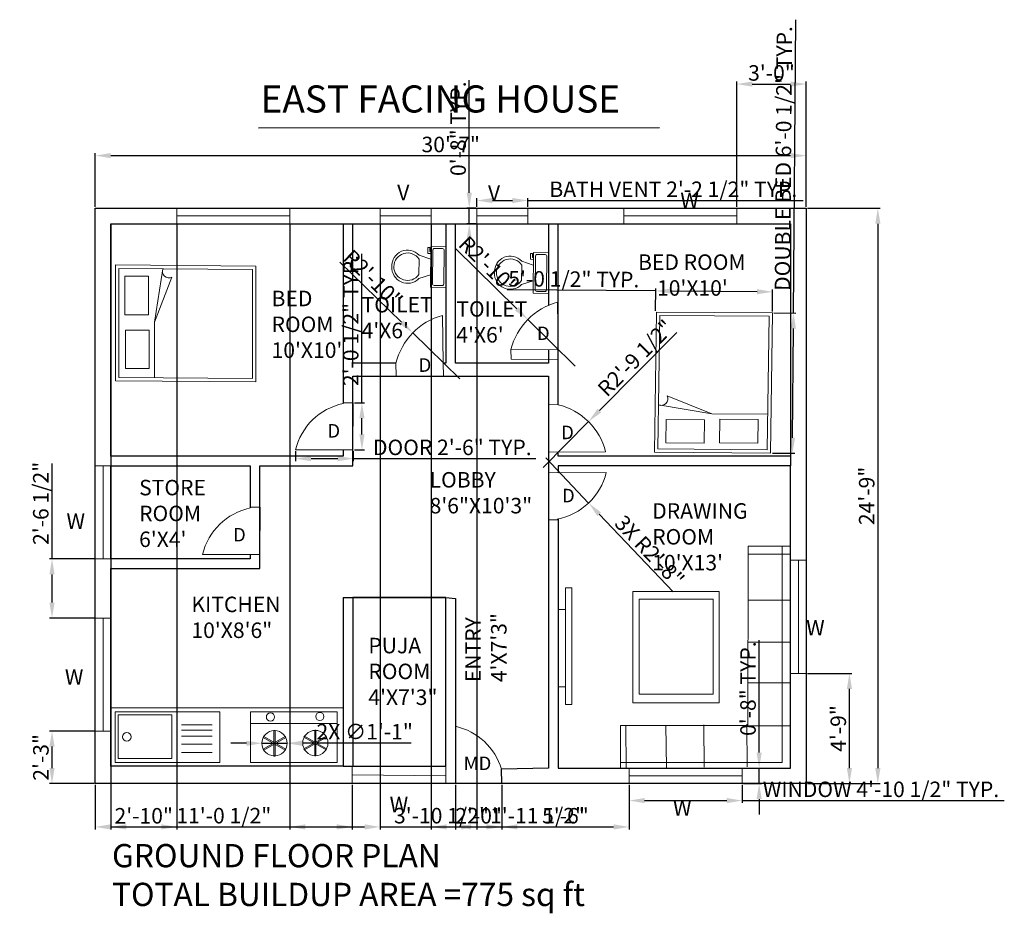
# Model space of a CAD drawing. Units: inches. Extents: x 853 to 1361, y 275 to 736.
import ezdxf

# ---------------------------------------------------------------- set-up
doc = ezdxf.new("R2010")
doc.units = ezdxf.units.IN
for name, color, linetype, lineweight in [('A-ANNO-DIMS', 2, 'Continuous', 18), ('A-ANNO-TEXT', 7, 'Continuous', 18), ('A-ANNO-TTLB', 7, 'Continuous', 30), ('A-AREA-IDEN', 7, 'Continuous', 18), ('A-DOOR', 3, 'Continuous', 18), ('A-EQPM', 8, 'Continuous', 18), ('A-FLOR-FIXT', 9, 'Continuous', 18), ('A-FURN', 8, 'Continuous', 18), ('A-GLAZ', 4, 'Continuous', 18), ('A-WALL', 7, 'Continuous', 30)]:
    doc.layers.add(name, color=color, linetype=linetype, lineweight=lineweight)
doc.styles.get("Standard").update_dxf_attribs({"font": 'arial.ttf'})
doc.dimstyles.new('ISO-25', dxfattribs={"dimtxt": 8, "dimasz": 8, "dimexe": 1.25, "dimexo": 0.625, "dimtad": 1, "dimlunit": 3, "dimtxsty": 'Standard', "dimcen": 2.5, "dimadec": 0, "dimazin": 0, "dimtfac": 1, "dimtmove": 0, "dimatfit": 3, "dimfxl": 1, "dimarcsym": 0})

# ---------------------------------------------------------------- blocks, each defined once
blk = doc.blocks.new('*U2')
for p, q in [((9.5, -6), (9.5, -2)), ((-10, -8.5), (-8, -8.5)), ((-10, -9.5), (-10, -8.5)), ((-7, -9.5), (-10, -9.5)), ((-8, -8.5), (-8, -8)), ((-7, -8), (-7, -9.5)), ((-4, -8), (-6, -14)), ((4, -8), (6, -14)), ((4, -14), (-4, -14))]:
    blk.add_line(p, q)
blk.add_lwpolyline([(10.5, -8), (10.5, 0), (-10.5, 0), (-10.5, -8)], close=True)
for points in [[(-9.5, -2), (-9.5, -6)], [(8.5, -1), (-8.5, -1)], [(-8.5, -7), (8.5, -7)]]:
    blk.add_lwpolyline(points)
for centre, radius, start, end in [((-8.625, -1.875), 0.8839, 81.8699, 188.1301), ((8.625, -1.875), 0.8839, 351.8699, 98.1301), ((-8.625, -6.125), 0.8839, 171.869898, 278.1301), ((8.625, -6.125), 0.8839, 261.8699, 8.1301), ((-0.4772, -19.9188), 8.0953, 133.01722, 273.38), ((0.0374, -19.8731), 7.127, 124.50543, 269.7), ((-0.0373, -19.8731), 7.127, 270.3, 55.4946), ((0.4773, -19.9188), 8.0953, 266.62, 46.9828)]:
    blk.add_arc(centre, radius, start, end)
blk = doc.blocks.new('*U3')
blk.add_lwpolyline([(-0.3, 3.29), (0.3, 3.29), (0.3, -3.29), (-0.3, -3.29)], close=True)
blk = doc.blocks.new('*U4')
at = {"layer": 'A-EQPM', "color": 0, "linetype": 'ByBlock', "lineweight": -2, "transparency": 16777216}
for p, rotation in [((981.29, 364.33), 59.99999999999999), ((986.99, 364.33), 300), ((981.29, 361.04), 120), ((984.14, 359.4), 180), ((986.99, 361.04), 240)]:
    blk.add_blockref('*U3', p, dxfattribs=dict(at, rotation=rotation))
blk.add_blockref('*U3', (984.14, 365.98), dxfattribs=at)
blk = doc.blocks.new('*U5')
blk.add_lwpolyline([(-0.3, 3.29), (0.3, 3.29), (0.3, -3.29), (-0.3, -3.29)], close=True)
blk = doc.blocks.new('*U6')
at = {"layer": 'A-EQPM', "color": 0, "linetype": 'ByBlock', "lineweight": -2, "transparency": 16777216}
for p, rotation in [((981.29, 364.33), 59.99999999999999), ((986.99, 364.33), 300), ((981.29, 361.04), 120), ((984.14, 359.4), 180), ((986.99, 361.04), 240)]:
    blk.add_blockref('*U5', p, dxfattribs=dict(at, rotation=rotation))
blk.add_blockref('*U5', (984.14, 365.98), dxfattribs=at)
blk = doc.blocks.new('*D7')
at = {"layer": 'A-ANNO-DIMS', "color": 0, "lineweight": -2, "transparency": 16777216}
for p, q in [((891.64, 639.56), (891.64, 667.31)), ((899.64, 666.06), (1250.64, 666.06)), ((1258.64, 639.56), (1258.64, 667.31))]:
    blk.add_line(p, q, dxfattribs=at)
at = {"layer": 'A-ANNO-DIMS', "color": 0, "transparency": 16777216}
for points in [[(899.64, 667.39), (899.64, 664.72), (891.64, 666.06)], [(1250.64, 667.39), (1250.64, 664.72), (1258.64, 666.06)]]:
    blk.add_solid(points, dxfattribs=at)
at = {"layer": 'Defpoints', "color": 0, "transparency": 16777216}
for p in [(1258.64, 666.06), (891.64, 638.93), (1258.64, 638.93)]:
    blk.add_point(p, dxfattribs=at)
at = {"layer": 'A-ANNO-DIMS', "color": 0, "transparency": 16777216, "insert": (1075.14, 670.77), "char_height": 8, "attachment_point": 5}
blk.add_mtext('30\'-7"', dxfattribs=at)
blk = doc.blocks.new('*D8')
at = {"layer": 'A-ANNO-DIMS', "color": 0, "lineweight": -2, "transparency": 16777216}
for p, q in [((1259.27, 638.93), (1296.91, 638.93)), ((1295.66, 630.93), (1295.66, 349.93)), ((1259.27, 341.93), (1296.91, 341.93))]:
    blk.add_line(p, q, dxfattribs=at)
at = {"layer": 'A-ANNO-DIMS', "color": 0, "transparency": 16777216}
for points in [[(1294.33, 630.93), (1297, 630.93), (1295.66, 638.93)], [(1294.33, 349.93), (1297, 349.93), (1295.66, 341.93)]]:
    blk.add_solid(points, dxfattribs=at)
at = {"layer": 'Defpoints', "color": 0, "transparency": 16777216}
for p in [(1258.64, 638.93), (1258.64, 341.93), (1295.66, 341.93)]:
    blk.add_point(p, dxfattribs=at)
at = {"layer": 'A-ANNO-DIMS', "color": 0, "transparency": 16777216, "insert": (1290.95, 490.43), "char_height": 8, "attachment_point": 5, "rotation": 90}
blk.add_mtext('24\'-9"', dxfattribs=at)
blk = doc.blocks.new('BED-DOUBLE')
for p, q in [((20.06, 30.94), (24.46, 58.45)), ((24.46, 58.45), (20.06, 30.94)), ((20.06, 30.94), (29.09, 54.06)), ((20.06, 2.13), (20.06, 30.94))]:
    blk.add_line(p, q)
for points in [[(0, 60.38), (72.37, 59.83), (72.37, 0), (0, 0.54)], [(1.74, 58.62), (70.63, 58.1), (70.63, 1.76), (1.74, 2.27)], [(4.8, 54.53), (16.95, 54.53), (16.95, 34.73), (4.8, 34.73)], [(5.09, 6.98), (17.24, 6.98), (17.24, 26.78), (5.09, 26.78)]]:
    blk.add_lwpolyline(points, close=True)
blk.add_arc((27.58, 57.1), 3.4, 156.697, 296.2108)
blk = doc.blocks.new('WINDOW-STANDARD')
blk.add_line((0, 4), (58.38, 4))
blk.add_lwpolyline([(0, 0), (58.38, 0), (58.38, 8), (0, 8)], close=True)
blk = doc.blocks.new('DOOR-SINGLE-INTERIOR')
blk.add_line((24.63, 0), (0, 0))
blk.add_lwpolyline([(24.63, 0), (29.63, 0), (29.82, 24.4), (24.82, 24.4)])
blk.add_arc((31.29, -7.54), 32.19, 101.9374, 166.4496)
blk = doc.blocks.new('VENT-BATH')
blk.add_line((0, 4), (26.34, 4))
blk.add_lwpolyline([(0, 8), (26.34, 8), (26.34, 0), (0, 0)], close=True)
blk = doc.blocks.new('*D13')
at = {"layer": 'A-ANNO-DIMS', "color": 0, "lineweight": -2, "transparency": 16777216}
for p, q in [((1167.24, 341.31), (1167.24, 331.93)), ((1225.62, 341.31), (1225.62, 331.93)), ((1175.24, 333.18), (1217.62, 333.18)), ((1225.62, 333.18), (1360.96, 333.18))]:
    blk.add_line(p, q, dxfattribs=at)
at = {"layer": 'A-ANNO-DIMS', "color": 0, "transparency": 16777216}
for points in [[(1175.24, 334.51), (1175.24, 331.84), (1167.24, 333.18)], [(1217.62, 334.51), (1217.62, 331.84), (1225.62, 333.18)]]:
    blk.add_solid(points, dxfattribs=at)
at = {"layer": 'Defpoints', "color": 0, "transparency": 16777216}
for p in [(1167.24, 341.93), (1225.62, 341.93), (1225.62, 333.18)]:
    blk.add_point(p, dxfattribs=at)
at = {"layer": 'A-ANNO-DIMS', "color": 0, "transparency": 16777216, "insert": (1297.29, 337.94), "char_height": 8, "attachment_point": 5}
blk.add_mtext('WINDOW 4\'-10 1/2" TYP.', dxfattribs=at)
blk = doc.blocks.new('*D14')
at = {"layer": 'A-ANNO-DIMS', "color": 0, "lineweight": -2, "transparency": 16777216}
for p, q in [((1234.38, 357.93), (1234.38, 415.95)), ((1226.24, 349.93), (1235.63, 349.93)), ((1234.38, 341.93), (1234.38, 349.93)), ((1226.24, 341.93), (1235.63, 341.93)), ((1234.38, 333.93), (1234.38, 325.93))]:
    blk.add_line(p, q, dxfattribs=at)
at = {"layer": 'A-ANNO-DIMS', "color": 0, "transparency": 16777216}
for points in [[(1233.04, 357.93), (1235.71, 357.93), (1234.38, 349.93)], [(1233.04, 333.93), (1235.71, 333.93), (1234.38, 341.93)]]:
    blk.add_solid(points, dxfattribs=at)
at = {"layer": 'Defpoints', "color": 0, "transparency": 16777216}
for p in [(1225.62, 349.93), (1234.38, 349.93), (1225.62, 341.93)]:
    blk.add_point(p, dxfattribs=at)
at = {"layer": 'A-ANNO-DIMS', "color": 0, "transparency": 16777216, "insert": (1229.67, 390.94), "char_height": 8, "attachment_point": 5, "rotation": 90}
blk.add_mtext('0\'-8" TYP.', dxfattribs=at)
blk = doc.blocks.new('*D15')
at = {"layer": 'A-ANNO-DIMS', "color": 0, "lineweight": -2, "transparency": 16777216}
for p, q in [((1252.11, 584.81), (1253.24, 736.21)), ((1241.88, 584.89), (1253.36, 584.8)), ((1251.63, 520.45), (1252.05, 576.81)), ((1241.34, 512.52), (1252.82, 512.44))]:
    blk.add_line(p, q, dxfattribs=at)
at = {"layer": 'A-ANNO-DIMS', "color": 0, "transparency": 16777216}
for points in [[(1250.71, 576.82), (1253.38, 576.8), (1252.11, 584.81)], [(1250.29, 520.46), (1252.96, 520.44), (1251.57, 512.45)]]:
    blk.add_solid(points, dxfattribs=at)
at = {"layer": 'Defpoints', "color": 0, "transparency": 16777216}
for p in [(1241.25, 584.89), (1252.11, 584.81), (1240.71, 512.53)]:
    blk.add_point(p, dxfattribs=at)
at = {"layer": 'A-ANNO-DIMS', "color": 0, "transparency": 16777216, "insert": (1247.94, 664.55), "char_height": 8, "attachment_point": 5, "rotation": 89.5713}
blk.add_mtext('DOUBLE BED 6\'-0 1/2" TYP.', dxfattribs=at)
blk = doc.blocks.new('*D16')
at = {"layer": 'A-ANNO-DIMS', "color": 0, "lineweight": -2, "transparency": 16777216}
for p, q in [((1180.96, 596.2), (1104.31, 596.77)), ((1180.88, 585.97), (1180.97, 597.45)), ((1233.33, 595.81), (1188.96, 596.14)), ((1241.26, 585.52), (1241.34, 597))]:
    blk.add_line(p, q, dxfattribs=at)
at = {"layer": 'A-ANNO-DIMS', "color": 0, "transparency": 16777216}
for points in [[(1188.97, 597.47), (1188.95, 594.81), (1180.96, 596.2)], [(1233.34, 597.14), (1233.32, 594.48), (1241.33, 595.75)]]:
    blk.add_solid(points, dxfattribs=at)
at = {"layer": 'Defpoints', "color": 0, "transparency": 16777216}
for p in [(1180.96, 596.2), (1180.88, 585.35), (1241.25, 584.89)]:
    blk.add_point(p, dxfattribs=at)
at = {"layer": 'A-ANNO-DIMS', "color": 0, "transparency": 16777216, "insert": (1138.67, 601.28), "char_height": 8, "attachment_point": 5, "rotation": 359.5713}
blk.add_mtext('5\'-0 1/2" TYP.', dxfattribs=at)
blk = doc.blocks.new('*D17')
at = {"layer": 'A-ANNO-DIMS', "color": 0, "lineweight": -2, "transparency": 16777216}
for p, q in [((995.01, 513.52), (995.01, 508.42)), ((1024.83, 513.52), (1024.83, 508.42)), ((1003.01, 509.67), (1016.83, 509.67)), ((1024.83, 509.67), (1119.08, 509.67))]:
    blk.add_line(p, q, dxfattribs=at)
at = {"layer": 'A-ANNO-DIMS', "color": 0, "transparency": 16777216}
for points in [[(1003.01, 511), (1003.01, 508.34), (995.01, 509.67)], [(1016.83, 511), (1016.83, 508.34), (1024.83, 509.67)]]:
    blk.add_solid(points, dxfattribs=at)
at = {"layer": 'Defpoints', "color": 0, "transparency": 16777216}
for p in [(995.01, 514.14), (1024.83, 514.14), (1024.83, 509.67)]:
    blk.add_point(p, dxfattribs=at)
at = {"layer": 'A-ANNO-DIMS', "color": 0, "transparency": 16777216, "insert": (1075.96, 514.44), "char_height": 8, "attachment_point": 5}
blk.add_mtext('DOOR 2\'-6" TYP.', dxfattribs=at)
blk = doc.blocks.new('*D18')
at = {"layer": 'A-ANNO-DIMS', "color": 0, "lineweight": -2, "transparency": 16777216}
for p, q in [((1029.31, 538.54), (1029.31, 615.34)), ((1025.46, 538.54), (1030.56, 538.54)), ((1029.31, 522.14), (1029.31, 530.54)), ((1025.46, 514.14), (1030.56, 514.14))]:
    blk.add_line(p, q, dxfattribs=at)
at = {"layer": 'A-ANNO-DIMS', "color": 0, "transparency": 16777216}
for points in [[(1027.97, 530.54), (1030.64, 530.54), (1029.31, 538.54)], [(1027.97, 522.14), (1030.64, 522.14), (1029.31, 514.14)]]:
    blk.add_solid(points, dxfattribs=at)
at = {"layer": 'Defpoints', "color": 0, "transparency": 16777216}
for p in [(1024.83, 538.54), (1029.31, 538.54), (1024.83, 514.14)]:
    blk.add_point(p, dxfattribs=at)
at = {"layer": 'A-ANNO-DIMS', "color": 0, "transparency": 16777216, "insert": (1024.55, 580.94), "char_height": 8, "attachment_point": 5, "rotation": 90}
blk.add_mtext('2\'-0 1/2" TYP.', dxfattribs=at)
blk = doc.blocks.new('*D19')
at = {"layer": 'A-ANNO-DIMS', "color": 0, "lineweight": -2, "transparency": 16777216}
for p, q in [((1088.66, 639.56), (1088.66, 644.14)), ((1096.66, 642.89), (1107, 642.89)), ((1115, 639.56), (1115, 644.14)), ((1115, 642.89), (1257.13, 642.89))]:
    blk.add_line(p, q, dxfattribs=at)
at = {"layer": 'A-ANNO-DIMS', "color": 0, "transparency": 16777216}
for points in [[(1096.66, 644.22), (1096.66, 641.55), (1088.66, 642.89)], [(1107, 644.22), (1107, 641.55), (1115, 642.89)]]:
    blk.add_solid(points, dxfattribs=at)
at = {"layer": 'Defpoints', "color": 0, "transparency": 16777216}
for p in [(1115, 642.89), (1088.66, 638.93), (1115, 638.93)]:
    blk.add_point(p, dxfattribs=at)
at = {"layer": 'A-ANNO-DIMS', "color": 0, "transparency": 16777216, "insert": (1190.06, 647.65), "char_height": 8, "attachment_point": 5}
blk.add_mtext('BATH VENT 2\'-2 1/2" TYP.', dxfattribs=at)
blk = doc.blocks.new('*D20')
at = {"layer": 'A-ANNO-DIMS', "color": 0, "lineweight": -2, "transparency": 16777216}
for p, q in [((1084.71, 646.93), (1084.71, 704.95)), ((1088.04, 638.93), (1083.46, 638.93)), ((1084.71, 630.93), (1084.71, 638.93)), ((1088.04, 630.93), (1083.46, 630.93)), ((1084.71, 622.93), (1084.71, 614.93))]:
    blk.add_line(p, q, dxfattribs=at)
at = {"layer": 'A-ANNO-DIMS', "color": 0, "transparency": 16777216}
for points in [[(1083.38, 646.93), (1086.04, 646.93), (1084.71, 638.93)], [(1083.38, 622.93), (1086.04, 622.93), (1084.71, 630.93)]]:
    blk.add_solid(points, dxfattribs=at)
at = {"layer": 'Defpoints', "color": 0, "transparency": 16777216}
for p in [(1084.71, 638.93), (1088.66, 638.93), (1088.66, 630.93)]:
    blk.add_point(p, dxfattribs=at)
at = {"layer": 'A-ANNO-DIMS', "color": 0, "transparency": 16777216, "insert": (1080, 679.94), "char_height": 8, "attachment_point": 5, "rotation": 90}
blk.add_mtext('0\'-8" TYP.', dxfattribs=at)
blk = doc.blocks.new('*D21')
at = {"layer": 'A-ANNO-DIMS', "color": 0, "lineweight": -2, "transparency": 16777216}
for p, q in [((899.64, 630.31), (899.64, 318.33)), ((933.66, 630.31), (933.66, 318.33)), ((907.64, 319.58), (925.66, 319.58))]:
    blk.add_line(p, q, dxfattribs=at)
at = {"layer": 'A-ANNO-DIMS', "color": 0, "transparency": 16777216}
for points in [[(907.64, 320.92), (907.64, 318.25), (899.64, 319.58)], [(925.66, 320.92), (925.66, 318.25), (933.66, 319.58)]]:
    blk.add_solid(points, dxfattribs=at)
at = {"layer": 'Defpoints', "color": 0, "transparency": 16777216}
for p in [(899.64, 630.93), (933.66, 630.93), (933.66, 319.58)]:
    blk.add_point(p, dxfattribs=at)
at = {"layer": 'A-ANNO-DIMS', "color": 0, "transparency": 16777216, "insert": (916.65, 324.29), "char_height": 8, "attachment_point": 5}
blk.add_mtext('2\'-10"', dxfattribs=at)
blk = doc.blocks.new('*D22')
at = {"layer": 'A-ANNO-DIMS', "color": 0, "lineweight": -2, "transparency": 16777216}
for p, q in [((992.04, 630.31), (992.04, 318.33)), ((1038.68, 630.31), (1038.68, 318.33)), ((1000.04, 319.58), (1030.68, 319.58)), ((1038.68, 319.58), (1094.05, 319.58))]:
    blk.add_line(p, q, dxfattribs=at)
at = {"layer": 'A-ANNO-DIMS', "color": 0, "transparency": 16777216}
for points in [[(1000.04, 320.92), (1000.04, 318.25), (992.04, 319.58)], [(1030.68, 320.92), (1030.68, 318.25), (1038.68, 319.58)]]:
    blk.add_solid(points, dxfattribs=at)
at = {"layer": 'Defpoints', "color": 0, "transparency": 16777216}
for p in [(992.04, 630.93), (1038.68, 630.93), (1038.68, 319.58)]:
    blk.add_point(p, dxfattribs=at)
at = {"layer": 'A-ANNO-DIMS', "color": 0, "transparency": 16777216, "insert": (1070.37, 324.35), "char_height": 8, "attachment_point": 5}
blk.add_mtext('3\'-10 1/2"', dxfattribs=at)
blk = doc.blocks.new('*D23')
at = {"layer": 'A-ANNO-DIMS', "color": 0, "lineweight": -2, "transparency": 16777216}
for p, q in [((1065.02, 630.31), (1065.02, 318.33)), ((1088.66, 630.31), (1088.66, 318.33)), ((1073.02, 319.58), (1080.66, 319.58)), ((1088.66, 319.58), (1143.28, 319.58))]:
    blk.add_line(p, q, dxfattribs=at)
at = {"layer": 'A-ANNO-DIMS', "color": 0, "transparency": 16777216}
for points in [[(1073.02, 320.92), (1073.02, 318.25), (1065.02, 319.58)], [(1080.66, 320.92), (1080.66, 318.25), (1088.66, 319.58)]]:
    blk.add_solid(points, dxfattribs=at)
at = {"layer": 'Defpoints', "color": 0, "transparency": 16777216}
for p in [(1065.02, 630.93), (1088.66, 630.93), (1088.66, 319.58)]:
    blk.add_point(p, dxfattribs=at)
at = {"layer": 'A-ANNO-DIMS', "color": 0, "transparency": 16777216, "insert": (1119.97, 324.35), "char_height": 8, "attachment_point": 5}
blk.add_mtext('1\'-11 1/2"', dxfattribs=at)
blk = doc.blocks.new('*D24')
at = {"layer": 'A-ANNO-DIMS', "color": 0, "lineweight": -2, "transparency": 16777216}
for p, q in [((1222.86, 639.56), (1222.86, 704.24)), ((1230.86, 702.99), (1250.64, 702.99)), ((1258.64, 639.56), (1258.64, 704.24))]:
    blk.add_line(p, q, dxfattribs=at)
at = {"layer": 'A-ANNO-DIMS', "color": 0, "transparency": 16777216}
for points in [[(1230.86, 704.32), (1230.86, 701.65), (1222.86, 702.99)], [(1250.64, 704.32), (1250.64, 701.65), (1258.64, 702.99)]]:
    blk.add_solid(points, dxfattribs=at)
at = {"layer": 'Defpoints', "color": 0, "transparency": 16777216}
for p in [(1258.64, 702.99), (1222.86, 638.93), (1258.64, 638.93)]:
    blk.add_point(p, dxfattribs=at)
at = {"layer": 'A-ANNO-DIMS', "color": 0, "transparency": 16777216, "insert": (1240.75, 707.7), "char_height": 8, "attachment_point": 5}
blk.add_mtext('3\'-0"', dxfattribs=at)
blk = doc.blocks.new('*D25')
at = {"layer": 'A-ANNO-DIMS', "color": 0, "lineweight": -2, "transparency": 16777216}
for p, q in [((891.02, 369), (868.04, 369)), ((869.29, 349.93), (869.29, 361)), ((891.02, 341.93), (868.04, 341.93))]:
    blk.add_line(p, q, dxfattribs=at)
at = {"layer": 'A-ANNO-DIMS', "color": 0, "transparency": 16777216}
for points in [[(867.96, 361), (870.63, 361), (869.29, 369)], [(867.96, 349.93), (870.63, 349.93), (869.29, 341.93)]]:
    blk.add_solid(points, dxfattribs=at)
at = {"layer": 'Defpoints', "color": 0, "transparency": 16777216}
for p in [(869.29, 369), (891.64, 369), (891.64, 341.93)]:
    blk.add_point(p, dxfattribs=at)
at = {"layer": 'A-ANNO-DIMS', "color": 0, "transparency": 16777216, "insert": (864.58, 355.47), "char_height": 8, "attachment_point": 5, "rotation": 90}
blk.add_mtext('2\'-3"', dxfattribs=at)
blk = doc.blocks.new('*D26')
at = {"layer": 'A-ANNO-DIMS', "color": 0, "lineweight": -2, "transparency": 16777216}
for p, q in [((869.29, 457.93), (869.29, 507.23)), ((891.02, 457.93), (868.04, 457.93)), ((869.29, 435.38), (869.29, 449.93)), ((891.02, 427.38), (868.04, 427.38))]:
    blk.add_line(p, q, dxfattribs=at)
at = {"layer": 'A-ANNO-DIMS', "color": 0, "transparency": 16777216}
for points in [[(867.96, 449.93), (870.63, 449.93), (869.29, 457.93)], [(867.96, 435.38), (870.63, 435.38), (869.29, 427.38)]]:
    blk.add_solid(points, dxfattribs=at)
at = {"layer": 'Defpoints', "color": 0, "transparency": 16777216}
for p in [(869.29, 457.93), (891.64, 457.93), (891.64, 427.38)]:
    blk.add_point(p, dxfattribs=at)
at = {"layer": 'A-ANNO-DIMS', "color": 0, "transparency": 16777216, "insert": (864.53, 486.58), "char_height": 8, "attachment_point": 5, "rotation": 90}
blk.add_mtext('2\'-6 1/2"', dxfattribs=at)
blk = doc.blocks.new('*D27')
at = {"layer": 'A-ANNO-DIMS', "color": 0, "lineweight": -2, "transparency": 16777216}
for p, q in [((1259.27, 398.84), (1282.24, 398.84)), ((1280.99, 349.93), (1280.99, 390.84)), ((1259.27, 341.93), (1282.24, 341.93))]:
    blk.add_line(p, q, dxfattribs=at)
at = {"layer": 'A-ANNO-DIMS', "color": 0, "transparency": 16777216}
for points in [[(1279.66, 390.84), (1282.33, 390.84), (1280.99, 398.84)], [(1279.66, 349.93), (1282.33, 349.93), (1280.99, 341.93)]]:
    blk.add_solid(points, dxfattribs=at)
at = {"layer": 'Defpoints', "color": 0, "transparency": 16777216}
for p in [(1258.64, 398.84), (1280.99, 398.84), (1258.64, 341.93)]:
    blk.add_point(p, dxfattribs=at)
at = {"layer": 'A-ANNO-DIMS', "color": 0, "transparency": 16777216, "insert": (1276.28, 370.39), "char_height": 8, "attachment_point": 5, "rotation": 90}
blk.add_mtext('4\'-9"', dxfattribs=at)
blk = doc.blocks.new('*D28')
at = {"layer": 'A-ANNO-DIMS', "color": 0, "lineweight": -2, "transparency": 16777216}
for p, q in [((891.64, 341.31), (891.64, 318.33)), ((1024.34, 341.31), (1024.34, 318.33)), ((899.64, 319.58), (1016.34, 319.58))]:
    blk.add_line(p, q, dxfattribs=at)
at = {"layer": 'A-ANNO-DIMS', "color": 0, "transparency": 16777216}
for points in [[(899.64, 320.92), (899.64, 318.25), (891.64, 319.58)], [(1016.34, 320.92), (1016.34, 318.25), (1024.34, 319.58)]]:
    blk.add_solid(points, dxfattribs=at)
at = {"layer": 'Defpoints', "color": 0, "transparency": 16777216}
for p in [(891.64, 341.93), (1024.34, 341.93), (1024.34, 319.58)]:
    blk.add_point(p, dxfattribs=at)
at = {"layer": 'A-ANNO-DIMS', "color": 0, "transparency": 16777216, "insert": (957.99, 324.35), "char_height": 8, "attachment_point": 5}
blk.add_mtext('11\'-0 1/2"', dxfattribs=at)
blk = doc.blocks.new('*D29')
at = {"layer": 'A-ANNO-DIMS', "color": 0, "lineweight": -2, "transparency": 16777216}
for p, q in [((1077.62, 341.31), (1077.62, 318.33)), ((1101.48, 341.31), (1101.48, 318.33)), ((1085.62, 319.58), (1093.48, 319.58))]:
    blk.add_line(p, q, dxfattribs=at)
at = {"layer": 'A-ANNO-DIMS', "color": 0, "transparency": 16777216}
for points in [[(1085.62, 320.92), (1085.62, 318.25), (1077.62, 319.58)], [(1093.48, 320.92), (1093.48, 318.25), (1101.48, 319.58)]]:
    blk.add_solid(points, dxfattribs=at)
at = {"layer": 'Defpoints', "color": 0, "transparency": 16777216}
for p in [(1077.62, 341.93), (1101.48, 341.93), (1101.48, 319.58)]:
    blk.add_point(p, dxfattribs=at)
at = {"layer": 'A-ANNO-DIMS', "color": 0, "transparency": 16777216, "insert": (1089.55, 324.29), "char_height": 8, "attachment_point": 5}
blk.add_mtext('2\'-0"', dxfattribs=at)
blk = doc.blocks.new('*D30')
at = {"layer": 'A-ANNO-DIMS', "color": 0, "lineweight": -2, "transparency": 16777216}
for p, q in [((1101.48, 341.31), (1101.48, 318.33)), ((1167.24, 341.31), (1167.24, 318.33)), ((1109.48, 319.58), (1159.24, 319.58))]:
    blk.add_line(p, q, dxfattribs=at)
at = {"layer": 'A-ANNO-DIMS', "color": 0, "transparency": 16777216}
for points in [[(1109.48, 320.92), (1109.48, 318.25), (1101.48, 319.58)], [(1159.24, 320.92), (1159.24, 318.25), (1167.24, 319.58)]]:
    blk.add_solid(points, dxfattribs=at)
at = {"layer": 'Defpoints', "color": 0, "transparency": 16777216}
for p in [(1101.48, 341.93), (1167.24, 341.93), (1167.24, 319.58)]:
    blk.add_point(p, dxfattribs=at)
at = {"layer": 'A-ANNO-DIMS', "color": 0, "transparency": 16777216, "insert": (1134.36, 324.29), "char_height": 8, "attachment_point": 5}
blk.add_mtext('5\'-6"', dxfattribs=at)
blk = doc.blocks.new('*D31')
at = {"layer": 'A-ANNO-DIMS', "color": 0, "lineweight": -2, "transparency": 16777216}
for p, q in [((1077.62, 618.2), (1109.24, 587.05)), ((1139.31, 557.44), (1114.94, 581.44))]:
    blk.add_line(p, q, dxfattribs=at)
at = {"layer": 'A-ANNO-DIMS', "color": 0, "transparency": 16777216}
blk.add_solid([(1110.18, 588), (1108.31, 586.1), (1114.94, 581.44)], dxfattribs=at)
at = {"layer": 'Defpoints', "color": 0, "transparency": 16777216}
for p in [(1114.94, 581.44), (1139.31, 557.44)]:
    blk.add_point(p, dxfattribs=at)
at = {"layer": 'A-ANNO-DIMS', "color": 0, "transparency": 16777216, "insert": (1093.88, 608.79), "char_height": 8, "attachment_point": 5, "rotation": 315.4369}
blk.add_mtext('R2\'-10"', dxfattribs=at)
blk = doc.blocks.new('*D32')
at = {"layer": 'A-ANNO-DIMS', "color": 0, "lineweight": -2, "transparency": 16777216}
for p, q in [((1017.97, 611.08), (1049.79, 580.13)), ((1079.83, 550.89), (1055.52, 574.55))]:
    blk.add_line(p, q, dxfattribs=at)
at = {"layer": 'A-ANNO-DIMS', "color": 0, "transparency": 16777216}
blk.add_solid([(1050.72, 581.08), (1048.86, 579.17), (1055.52, 574.55)], dxfattribs=at)
at = {"layer": 'Defpoints', "color": 0, "transparency": 16777216}
for p in [(1055.52, 574.55), (1079.83, 550.89)]:
    blk.add_point(p, dxfattribs=at)
at = {"layer": 'A-ANNO-DIMS', "color": 0, "transparency": 16777216, "insert": (1034.3, 601.77), "char_height": 8, "attachment_point": 5, "rotation": 315.7852}
blk.add_mtext('R2\'-10"', dxfattribs=at)
blk = doc.blocks.new('*D33')
at = {"layer": 'A-ANNO-DIMS', "color": 0, "lineweight": -2, "transparency": 16777216}
for p, q in [((1191.85, 574.81), (1151.88, 534.44)), ((1122.8, 505.06), (1146.25, 528.75))]:
    blk.add_line(p, q, dxfattribs=at)
at = {"layer": 'A-ANNO-DIMS', "color": 0, "transparency": 16777216}
blk.add_solid([(1150.93, 535.37), (1152.83, 533.5), (1146.25, 528.75)], dxfattribs=at)
at = {"layer": 'Defpoints', "color": 0, "transparency": 16777216}
for p in [(1146.25, 528.75), (1122.8, 505.06)]:
    blk.add_point(p, dxfattribs=at)
at = {"layer": 'A-ANNO-DIMS', "color": 0, "transparency": 16777216, "insert": (1171.3, 560.82), "char_height": 8, "attachment_point": 5, "rotation": 45.287}
blk.add_mtext('R2\'-9 1/2"', dxfattribs=at)
blk = doc.blocks.new('*D34')
at = {"layer": 'A-ANNO-DIMS', "color": 0, "lineweight": -2, "transparency": 16777216}
for p, q in [((1124.17, 510.09), (1146.33, 486.76)), ((1189.98, 440.83), (1151.85, 480.96))]:
    blk.add_line(p, q, dxfattribs=at)
at = {"layer": 'A-ANNO-DIMS', "color": 0, "transparency": 16777216}
blk.add_solid([(1152.81, 481.88), (1150.88, 480.04), (1146.33, 486.76)], dxfattribs=at)
at = {"layer": 'Defpoints', "color": 0, "transparency": 16777216}
for p in [(1124.17, 510.09), (1146.33, 486.76)]:
    blk.add_point(p, dxfattribs=at)
at = {"layer": 'A-ANNO-DIMS', "color": 0, "transparency": 16777216, "insert": (1177.08, 461.24), "char_height": 8, "attachment_point": 5, "rotation": 313.5358}
blk.add_mtext('3X R2\'-8"', dxfattribs=at)
blk = doc.blocks.new('*D35')
at = {"layer": 'A-ANNO-DIMS', "color": 0, "lineweight": -2, "transparency": 16777216}
for p, q in [((969.62, 362.74), (961.62, 362.74)), ((977.62, 362.75), (990.66, 362.75)), ((1054.78, 362.75), (998.66, 362.75))]:
    blk.add_line(p, q, dxfattribs=at)
at = {"layer": 'A-ANNO-DIMS', "color": 0, "transparency": 16777216}
for points in [[(969.62, 364.08), (969.62, 361.41), (977.62, 362.75)], [(998.66, 364.08), (998.66, 361.41), (990.66, 362.75)]]:
    blk.add_solid(points, dxfattribs=at)
at = {"layer": 'Defpoints', "color": 0, "transparency": 16777216}
for p in [(977.62, 362.75), (990.66, 362.75)]:
    blk.add_point(p, dxfattribs=at)
at = {"layer": 'A-ANNO-DIMS', "color": 0, "transparency": 16777216, "insert": (1030.72, 367.68), "char_height": 8, "attachment_point": 5, "rotation": 0.0035}
blk.add_mtext('2X ∅1\'-1"', dxfattribs=at)

msp = doc.modelspace()

# ---------------------------------------------------------------- linework, layer by layer
at = {"layer": 'A-ANNO-TTLB'}
for p, q in [((975.963, 680.472), (1182.887, 680.635)), ((1179.822, 680.633), (1179.822, 680.633)), ((1179.822, 680.633), (1179.822, 680.633))]:
    msp.add_line(p, q, dxfattribs=at)
at = {"layer": 'A-DOOR'}
for p, q in [((1130.606, 565.783), (1130.235, 590.413)), ((1071.278, 558.988), (1070.907, 583.618)), ((1130.643, 513.056), (1155.117, 513.23)), ((1130.643, 502.394), (1155.459, 502.567)), ((1077.616, 346.836), (1077.616, 371.5))]:
    msp.add_line(p, q, dxfattribs=at)
msp.add_lwpolyline([(1130.606, 565.783), (1130.681, 560.784), (1106.275, 561.009), (1106.2, 566.009)], close=True, dxfattribs=at)
for points in [[(1071.278, 558.988), (1071.353, 552.245), (1046.952, 552.177), (1046.877, 558.92)], [(1130.643, 513.056), (1125.644, 513.156), (1125.657, 537.559), (1130.656, 537.46), (1130.656, 537.457)], [(1130.643, 502.394), (1125.645, 502.512), (1125.645, 478.124), (1130.643, 478.124), (1130.643, 478.563)]]:
    msp.add_lwpolyline(points, dxfattribs=at)
for centre, radius, start, end in [((1139.309, 557.439), 34.2, 105.38691, 165.48778), ((1079.835, 550.893), 33.921, 105.25925, 166.31098), ((1122.801, 505.064), 33.332, 14.18079, 76.39244), ((1124.165, 510.09), 32.186, 280.58859, 346.48357), ((1070.547, 340.101), 32.186, 16.68525, 77.31259)]:
    msp.add_arc(centre, radius, start, end, dxfattribs=at)
at = {"layer": 'A-EQPM'}
msp.add_line((971.819, 372.938), (1016.476, 372.938), dxfattribs=at)
msp.add_lwpolyline([(971.819, 378.948), (1016.476, 378.948), (1016.476, 352.822), (971.819, 352.822)], close=True, dxfattribs=at)
for centre, radius in [((982.066, 376.325), 2.123), ((1007.549, 376.563), 2.124), ((984.142, 362.746), 6.519), ((1005.234, 362.873), 6.519)]:
    msp.add_circle(centre, radius, dxfattribs=at)
at = {"layer": 'A-FLOR-FIXT'}
for p, q in [((899.643, 381.024), (1019.643, 381.024)), ((936.171, 372.265), (951.972, 372.265)), ((936.094, 369.556), (951.894, 369.556)), ((936.094, 366.46), (951.894, 366.46)), ((936.094, 362.281), (951.894, 362.281)), ((936.094, 357.947), (951.894, 357.947))]:
    msp.add_line(p, q, dxfattribs=at)
for points in [[(901.851, 379.023), (955.849, 379.023), (955.849, 352.76), (901.851, 352.76)], [(903.461, 377.351), (931.134, 377.351), (931.134, 354.95), (903.461, 354.95)]]:
    msp.add_lwpolyline(points, close=True, dxfattribs=at)
msp.add_circle((907.956, 366.042), 2.196, dxfattribs=at)
at = {"layer": 'A-FURN'}
for p, q in [((1228.716, 464.564), (1228.709, 460.306)), ((1228.709, 460.306), (1228.709, 464.564)), ((1228.709, 464.564), (1246.235, 464.564)), ((1250.643, 464.564), (1228.716, 464.564)), ((1246.235, 460.306), (1246.235, 464.564)), ((1246.235, 464.564), (1250.643, 464.564)), ((1246.235, 464.564), (1246.235, 352.87)), ((1228.566, 371.841), (1228.709, 460.306)), ((1228.709, 460.306), (1250.643, 460.306)), ((1246.235, 352.87), (1246.235, 460.306)), ((1228.709, 436.61), (1250.643, 436.61)), ((1228.709, 414.861), (1250.643, 414.861)), ((1228.709, 393.982), (1250.643, 393.982)), ((1162.774, 371.841), (1165.509, 371.873)), ((1162.774, 349.935), (1162.774, 371.841)), ((1165.509, 371.841), (1164.278, 371.841)), ((1165.769, 349.935), (1165.509, 371.841)), ((1165.509, 371.841), (1228.566, 371.841)), ((1186.497, 350.181), (1186.238, 372.087)), ((1206.058, 350.413), (1205.798, 372.319)), ((1228.271, 350.676), (1228.011, 372.582)), ((1228.709, 371.798), (1250.643, 371.798)), ((1165.652, 369.531), (1165.652, 369.531)), ((1164.278, 352.87), (1162.774, 352.87)), ((1162.774, 352.87), (1162.774, 349.935)), ((1246.235, 352.87), (1164.278, 352.87))]:
    msp.add_line(p, q, dxfattribs=at)
for points in [[(1134.396, 442.962), (1137.662, 442.962), (1137.662, 382.746), (1134.396, 382.746)], [(1169.216, 441.132), (1213.707, 441.132), (1213.707, 383.649), (1169.216, 383.649)], [(1172.45, 437.066), (1210.645, 437.066), (1210.645, 388.098), (1172.45, 388.098)], [(1130.643, 431.713), (1134.396, 431.713), (1134.396, 391.966), (1130.643, 391.966)]]:
    msp.add_lwpolyline(points, close=True, dxfattribs=at)
at = {"layer": 'A-GLAZ'}
for p, q in [((895.643, 457.935), (895.643, 505.935)), ((1024.343, 346.435), (1072.643, 345.935))]:
    msp.add_line(p, q, dxfattribs=at)
for points in [[(899.643, 457.935), (899.643, 505.935), (891.643, 505.935), (891.643, 457.935)], [(1024.343, 341.935), (1072.643, 341.935), (1072.643, 350.935), (1024.343, 350.935)]]:
    msp.add_lwpolyline(points, close=True, dxfattribs=at)
at = {"layer": 'A-WALL'}
for p, q in [((891.643, 341.935), (891.643, 638.935)), ((891.643, 638.935), (899.643, 638.935)), ((899.643, 638.935), (1250.643, 638.935)), ((1250.643, 638.935), (1258.643, 638.935)), ((1258.643, 638.935), (1258.643, 349.935)), ((1019.643, 630.935), (1024.643, 630.935)), ((1072.643, 630.935), (1077.643, 630.935)), ((1125.643, 630.935), (1130.643, 630.935)), ((1024.579, 505.917), (1024.595, 552.224)), ((1024.595, 552.224), (1125.664, 552.187)), ((1125.664, 552.187), (1125.664, 349.935)), ((899.643, 510.935), (899.643, 505.935)), ((1250.643, 510.935), (1250.643, 505.935)), ((976.586, 452.935), (976.605, 505.935)), ((976.605, 505.935), (1024.579, 505.917)), ((1019.643, 438.022), (1072.643, 438.022)), ((1072.643, 438.022), (1077.616, 437.502)), ((1077.616, 437.502), (1077.616, 341.935)), ((1019.643, 350.935), (1024.643, 350.935)), ((1077.616, 346.836), (1077.616, 341.935)), ((1125.664, 349.935), (1101.378, 349.341)), ((1101.482, 341.935), (1101.378, 349.341)), ((1258.643, 349.935), (1258.643, 341.935)), ((899.643, 341.935), (891.643, 341.935)), ((1258.643, 341.935), (899.643, 341.935))]:
    msp.add_line(p, q, dxfattribs=at)
for points in [[(1019.643, 514.145), (1019.643, 510.935), (899.643, 510.935), (899.643, 630.935), (1019.643, 630.935), (1019.643, 538.093)], [(1046.881, 558.935), (1024.643, 558.935), (1024.643, 630.935), (1072.643, 630.935), (1072.643, 558.935), (1071.279, 558.935)], [(1125.643, 565.829), (1125.643, 558.935), (1077.643, 558.935), (1077.643, 630.935), (1125.643, 630.935), (1125.643, 588.79)], [(1130.643, 537.46), (1130.643, 630.935), (1250.643, 630.935), (1250.643, 510.935), (1130.643, 510.935), (1130.643, 513.056)], [(971.643, 460.245), (971.643, 457.935), (899.643, 457.935), (899.643, 505.935), (971.643, 505.935), (971.643, 484.193)], [(1130.643, 478.563), (1130.643, 349.935), (1250.643, 349.935), (1250.643, 505.935), (1130.643, 505.935), (1130.643, 502.394)], [(1019.643, 438.022), (1019.643, 350.935), (899.643, 350.935), (899.643, 452.935), (976.586, 452.935)]]:
    msp.add_lwpolyline(points, dxfattribs=at)
msp.add_lwpolyline([(1024.643, 350.935), (1072.643, 350.935), (1072.643, 437.935), (1024.643, 437.935)], close=True, dxfattribs=at)

# ---------------------------------------------------------------- block references
at = {"layer": 'A-DOOR'}
for p in [(995.011, 514.145), (947.011, 460.245)]:
    msp.add_blockref('DOOR-SINGLE-INTERIOR', p, dxfattribs=at)
at = {"layer": 'A-EQPM'}
for name, p in [('*U4', (0, 0)), ('*U6', (21.094, 0.17))]:
    msp.add_blockref(name, p, dxfattribs=at)
at = {"layer": 'A-FLOR-FIXT', "rotation": 269.4127374034051}
for p in [(1072.751, 608.521), (1125.751, 605.434)]:
    msp.add_blockref('*U2', p, dxfattribs=at)
at = {"layer": 'A-FURN'}
msp.add_blockref('BED-DOUBLE', (902.126, 549.234), dxfattribs=at)
at = {"layer": 'A-FURN', "rotation": 89.57132702119947}
msp.add_blockref('BED-DOUBLE', (1240.711, 512.527), dxfattribs=at)
at = {"layer": 'A-GLAZ'}
for name, p in [('WINDOW-STANDARD', (933.662, 630.935)), ('VENT-BATH', (1038.684, 630.935)), ('VENT-BATH', (1088.662, 630.935)), ('WINDOW-STANDARD', (1164.482, 630.935)), ('WINDOW-STANDARD', (1167.235, 341.935))]:
    msp.add_blockref(name, p, dxfattribs=at)
for p, rotation in [((1258.643, 398.842), 90), ((899.643, 368.996), 89.9999999999996)]:
    msp.add_blockref('WINDOW-STANDARD', p, dxfattribs=dict(at, rotation=rotation))

# ---------------------------------------------------------------- texts
at = {"layer": 'A-ANNO-TEXT', "attachment_point": 1}
for s, width, insert, char_height in [('V', 22.78416, (1047.526, 651.031), 8), ('V', 22.78416, (1094.364, 650.803), 8), ('W', 22.78416, (1193.674, 646.935), 8), ('D', 13.05455, (1119.662, 577.847), 7), ('D', 13.05455, (1058.551, 561.461), 7), ('D', 13.05455, (1011.48, 527.507), 7), ('D', 13.05455, (1132.165, 526.696), 7), ('D', 13.05455, (1132.605, 494.092), 7), ('W', 22.78416, (876.75, 481.386), 8), ('D', 13.05455, (962.771, 473.895), 7), ('W', 22.78416, (1258.643, 426.411), 8), ('W', 22.78416, (875.921, 400.989), 8), ('MD', 13.05455, (1081.796, 355.907), 7), ('W', 22.78416, (1043.605, 335.121), 8), ('W', 22.78416, (1189.896, 333.388), 8)]:
    msp.add_mtext_dynamic_manual_height_columns(s, width=width, gutter_width=12.5, heights=[0], dxfattribs=dict(at, insert=insert, char_height=char_height))
at = {"layer": 'A-ANNO-TTLB', "attachment_point": 1}
for s, width, insert, char_height in [('{\\fArial|b1|i0|c0|p34;\\H1.75x;EAST FACING HOUSE}', 228.93159, (976.981, 702.3), 8), ('{\\fArial|b1|i0|c0|p34;GROUND FLOOR PLAN\\P}TOTAL BUILDUP AREA =775 sq ft', 261.70173, (900.258, 310.746), 12)]:
    msp.add_mtext_dynamic_manual_height_columns(s, width=width, gutter_width=12.5, heights=[0], dxfattribs=dict(at, insert=insert, char_height=char_height))
at = {"layer": 'A-AREA-IDEN', "char_height": 12, "attachment_point": 1}
for s, width, insert in [("{\\H0.66667x;BED ROOM          10'X10'}", 68.0778, (1171.862, 615.088)), ("{\\H0.66667x;BED ROOM 10'X10'}", 36.57724, (982.635, 596.327)), ("{\\H0.66667x;TOILET\\P4'X6'}", 36.57724, (1029.116, 593.114)), ("{\\H0.66667x;TOILET\\P4'X6'}", 36.57724, (1078.037, 590.915)), ("{\\H0.66667x;STORE ROOM 6'X4'}", 36.57724, (914.255, 498.714)), ('{\\H0.66667x;LOBBY 8\'6"X10\'3"}', 36.57724, (1064.232, 502.734)), ("{\\H0.66667x;DRAWING \\PROOM\\P10'X13'}", 70.30136, (1179.157, 486.656)), ('{\\H0.66667x;KITCHEN\\P10\'X8\'6"}', 36.57724, (941.262, 438.424)), ('{\\H0.66667x;PUJA \\PROOM\\P4\'X7\'3"}', 36.57724, (1032.627, 417.179))]:
    msp.add_mtext_dynamic_manual_height_columns(s, width=width, gutter_width=12.5, heights=[0], dxfattribs=dict(at, insert=insert))
at = {"layer": 'A-AREA-IDEN', "insert": (1082.644, 394.285), "char_height": 12, "attachment_point": 1, "rotation": 90}
msp.add_mtext_dynamic_manual_height_columns('{\\H0.66667x;ENTRY 4\'X7\'3"}', width=36.57724, gutter_width=12.5, heights=[0], dxfattribs=at)

# ---------------------------------------------------------------- dimensions: what is measured, and where the dimension line sits
at = {"layer": 'A-ANNO-DIMS'}
for base, p1, p2, angle, text, picture, middle in [((1252.107, 584.813), (1240.711, 512.527), (1241.252, 584.894), 89.57133, 'DOUBLE BED <> TYP.', '*D15', (1247.94, 664.549)), ((1084.711, 638.935), (1088.662, 630.935), (1088.662, 638.935), 90, '<> TYP.', '*D20', (1080.002, 679.942)), ((1029.308, 538.544), (1024.835, 514.145), (1024.835, 538.544), 90, '<> TYP.', '*D18', (1024.547, 580.94)), ((1180.96, 596.201), (1241.252, 584.894), (1180.879, 585.346), 179.57133, '<> TYP.', '*D16', (1138.669, 601.279)), ((1234.375, 349.935), (1225.618, 341.935), (1225.618, 349.935), 90, '<> TYP.', '*D14', (1229.665, 390.942))]:
    dim = msp.add_linear_dim(base=base, p1=p1, p2=p2, angle=angle, text=text, dimstyle='ISO-25', override={"dimdec": 1, "dimlfac": 1, "dimrnd": 0, "dimzin": 1, "dimdsep": 46, "dimlunit": 4, "dimfrac": 2}, dxfattribs=at)
    dim.commit()
    dim.dimension.update_dxf_attribs({"geometry": picture, "text_midpoint": middle})
for base, p1, p2, override, picture, middle in [((1258.643, 702.985), (1222.865, 638.935), (1258.643, 638.935), {"dimdec": 1, "dimlfac": 1, "dimrnd": 0, "dimzin": 1, "dimdsep": 46, "dimlunit": 4, "dimfrac": 2}, '*D24', (1240.754, 707.697)), ((1258.643, 666.058), (891.643, 638.935), (1258.643, 638.935), {"dimclrd": 0, "dimclre": 0, "dimclrt": 0}, '*D7', (1075.143, 670.77)), ((933.662, 319.585), (899.643, 630.935), (933.662, 630.935), {"dimdec": 1, "dimlfac": 1, "dimrnd": 0, "dimzin": 1, "dimdsep": 46, "dimlunit": 4, "dimfrac": 2}, '*D21', (916.653, 324.294)), ((1038.684, 319.585), (992.044, 630.935), (1038.684, 630.935), {"dimdec": 1, "dimlfac": 1, "dimrnd": 0, "dimzin": 1, "dimdsep": 46, "dimlunit": 4, "dimfrac": 2}, '*D22', (1070.368, 324.349)), ((1088.662, 319.585), (1065.024, 630.935), (1088.662, 630.935), {"dimdec": 1, "dimlfac": 1, "dimrnd": 0, "dimzin": 1, "dimdsep": 46, "dimlunit": 4, "dimfrac": 2}, '*D23', (1119.972, 324.346)), ((1024.343, 319.585), (891.643, 341.935), (1024.343, 341.935), {"dimdec": 1, "dimlfac": 1, "dimrnd": 0, "dimzin": 1, "dimdsep": 46, "dimlunit": 4, "dimfrac": 2}, '*D28', (957.993, 324.346)), ((1101.482, 319.585), (1077.616, 341.935), (1101.482, 341.935), {"dimdec": 1, "dimlfac": 1, "dimrnd": 0, "dimzin": 1, "dimdsep": 46, "dimlunit": 4, "dimfrac": 2}, '*D29', (1089.549, 324.294)), ((1167.236, 319.585), (1101.482, 341.935), (1167.236, 341.935), {"dimdec": 1, "dimlfac": 1, "dimrnd": 0, "dimzin": 1, "dimdsep": 46, "dimlunit": 4, "dimfrac": 2}, '*D30', (1134.359, 324.294))]:
    dim = msp.add_linear_dim(base=base, p1=p1, p2=p2, dimstyle='ISO-25', override=override, dxfattribs=at)
    dim.commit()
    dim.dimension.update_dxf_attribs({"geometry": picture, "text_midpoint": middle})
for base, p1, p2, text, picture, middle in [((1115.002, 642.886), (1088.662, 638.935), (1115.002, 638.935), 'BATH VENT <> TYP.', '*D19', (1190.064, 647.647)), ((1024.835, 509.671), (995.011, 514.145), (1024.835, 514.145), 'DOOR <> TYP.', '*D17', (1075.959, 514.436)), ((1225.618, 333.177), (1167.236, 341.935), (1225.618, 341.935), 'WINDOW <> TYP.', '*D13', (1297.288, 337.942))]:
    dim = msp.add_linear_dim(base=base, p1=p1, p2=p2, text=text, dimstyle='ISO-25', override={"dimdec": 1, "dimlfac": 1, "dimrnd": 0, "dimzin": 1, "dimdsep": 46, "dimlunit": 4, "dimfrac": 2}, dxfattribs=at)
    dim.commit()
    dim.dimension.update_dxf_attribs({"geometry": picture, "text_midpoint": middle})
for base, p1, p2, override, picture, middle in [((1295.664, 341.935), (1258.643, 638.935), (1258.643, 341.935), {"dimclrd": 0, "dimclre": 0, "dimclrt": 0}, '*D8', (1290.955, 490.435)), ((869.293, 457.935), (891.643, 427.378), (891.643, 457.935), {"dimdec": 1, "dimlfac": 1, "dimrnd": 0, "dimzin": 1, "dimdsep": 46, "dimlunit": 4, "dimfrac": 2}, '*D26', (864.532, 486.581)), ((1280.993, 398.843), (1258.643, 341.935), (1258.643, 398.843), {"dimdec": 1, "dimlfac": 1, "dimrnd": 0, "dimzin": 1, "dimdsep": 46, "dimlunit": 4, "dimfrac": 2}, '*D27', (1276.284, 370.389)), ((869.293, 368.996), (891.643, 341.935), (891.643, 368.996), {"dimdec": 1, "dimlfac": 1, "dimrnd": 0, "dimzin": 1, "dimdsep": 46, "dimlunit": 4, "dimfrac": 2}, '*D25', (864.581, 355.465))]:
    dim = msp.add_linear_dim(base=base, p1=p1, p2=p2, angle=90, dimstyle='ISO-25', override=override, dxfattribs=at)
    dim.commit()
    dim.dimension.update_dxf_attribs({"geometry": picture, "text_midpoint": middle})
for center, mpoint, picture, middle in [((1139.309, 557.439), (1114.942, 581.437), '*D31', (1093.885, 608.786)), ((1079.835, 550.893), (1055.522, 574.548), '*D32', (1034.299, 601.768)), ((1122.801, 505.064), (1146.252, 528.751), '*D33', (1171.297, 560.815))]:
    dim = msp.add_radius_dim(center=center, mpoint=mpoint, dimstyle='ISO-25', override={"dimdec": 1, "dimlfac": 1, "dimrnd": 0, "dimzin": 1, "dimdsep": 46, "dimlunit": 4, "dimfrac": 2}, dxfattribs=at)
    dim.commit()
    dim.dimension.update_dxf_attribs({"geometry": picture, "text_midpoint": middle})
dim = msp.add_radius_dim(center=(1124.165, 510.09), mpoint=(1146.335, 486.757), text='3X <>', dimstyle='ISO-25', override={"dimdec": 1, "dimlfac": 1, "dimrnd": 0, "dimzin": 1, "dimdsep": 46, "dimlunit": 4, "dimfrac": 2}, dxfattribs=at)
dim.commit()
dim.dimension.update_dxf_attribs({"geometry": '*D34', "text_midpoint": (1177.082, 461.238)})
dim = msp.add_diameter_dim_2p(p1=(977.623, 362.745), p2=(990.661, 362.746), text='2X <>', dimstyle='ISO-25', override={"dimdec": 1, "dimlfac": 1, "dimrnd": 0, "dimzin": 1, "dimdsep": 46, "dimlunit": 4, "dimfrac": 2}, dxfattribs=at)
dim.commit()
dim.dimension.update_dxf_attribs({"geometry": '*D35', "text_midpoint": (1030.722, 362.748)})

doc.saveas('drawing.dxf')
